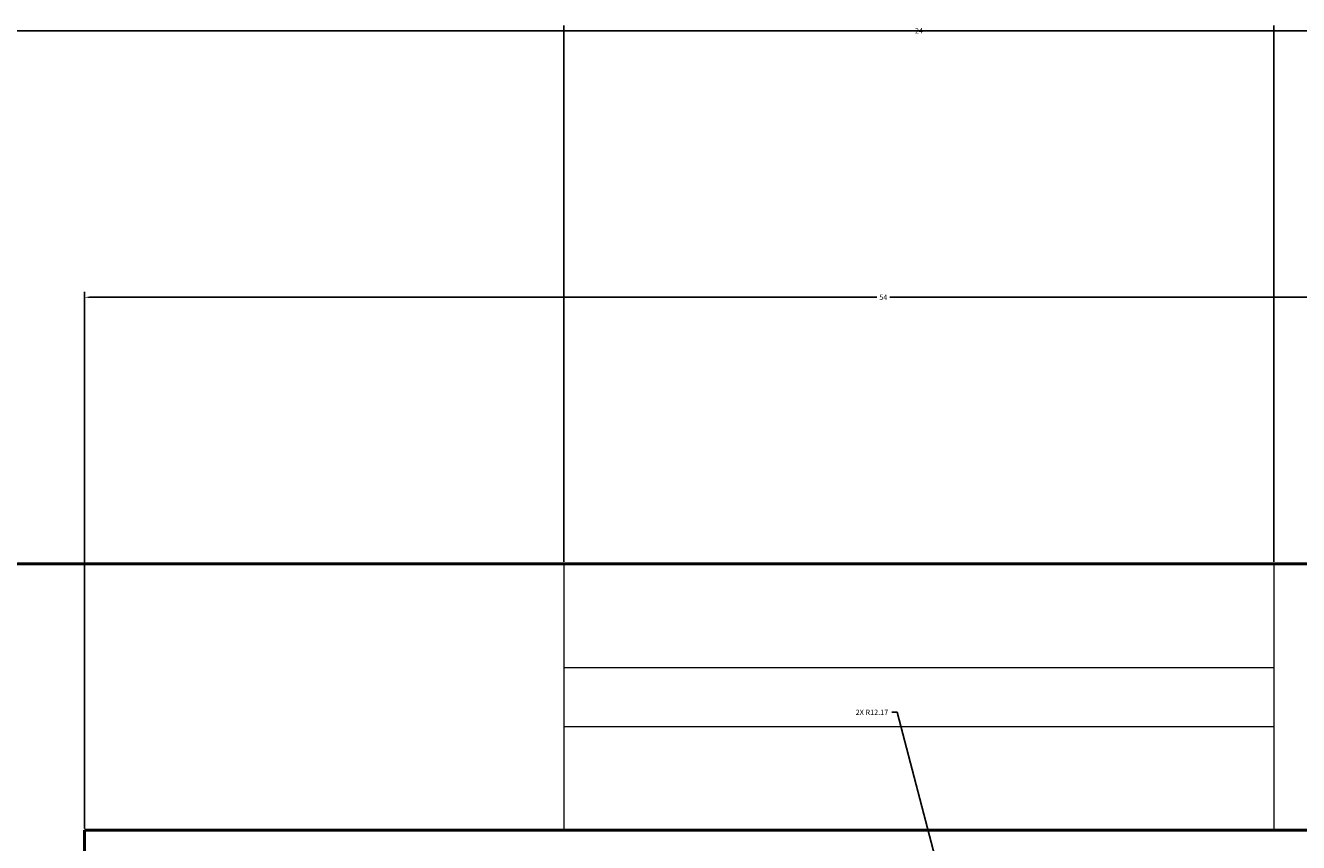
# Model space of a CAD drawing. Units: inches. Extents: x 2621 to 2849, y 2066 to 2463.
# Tile 26 of 28: x 2766 to 2809, y 2435 to 2463. Entities that reach past the tile are written whole.
import ezdxf

# ---------------------------------------------------------------- set-up
doc = ezdxf.new("R2010")
doc.units = ezdxf.units.IN
for name, color, linetype, lineweight in [('A-ANNO-DIMS', 2, 'Continuous', 18), ('A-GLAZ', 4, 'Continuous', 18), ('A-WALL', 7, 'Continuous', 50)]:
    doc.layers.add(name, color=color, linetype=linetype, lineweight=lineweight)
doc.styles.get("Standard").update_dxf_attribs({"font": 'arial.ttf'})
doc.dimstyles.get("Standard").update_dxf_attribs({"dimtxt": 0.18, "dimasz": 0.18, "dimexe": 0.18, "dimexo": 0.0625, "dimgap": 0.09, "dimtad": 0, "dimtih": 1, "dimtoh": 1, "dimdec": 4, "dimzin": 0, "dimdsep": 46, "dimtxsty": 'Standard', "dimcen": 0.09, "dimadec": 0, "dimazin": 0, "dimtfac": 1, "dimtdec": 4, "dimtofl": 0, "dimtmove": 0, "dimatfit": 3, "dimfxl": 1, "dimtolj": 1, "dimtzin": 0, "dimarcsym": 0})

# ---------------------------------------------------------------- blocks, each defined once
blk = doc.blocks.new('*D35')
at = {"layer": 'A-ANNO-DIMS', "color": 0, "lineweight": -2, "transparency": 16777216}
for p, q in [((2638.87, 2444.437), (2638.87, 2462.558)), ((2639.05, 2462.378), (2734.591, 2462.378)), ((2830.69, 2462.378), (2735.15, 2462.378)), ((2830.87, 2444.437), (2830.87, 2462.558))]:
    blk.add_line(p, q, dxfattribs=at)
at = {"layer": 'A-ANNO-DIMS', "color": 0, "transparency": 16777216}
for points in [[(2639.05, 2462.408), (2639.05, 2462.348), (2638.87, 2462.378)], [(2830.69, 2462.408), (2830.69, 2462.348), (2830.87, 2462.378)]]:
    blk.add_solid(points, dxfattribs=at)
at = {"layer": 'Defpoints', "color": 0, "transparency": 16777216}
for p in [(2830.87, 2462.378), (2638.87, 2444.375), (2830.87, 2444.375)]:
    blk.add_point(p, dxfattribs=at)
at = {"layer": 'A-ANNO-DIMS', "color": 0, "transparency": 16777216, "insert": (2734.87, 2462.378), "char_height": 0.18, "attachment_point": 5}
blk.add_mtext('\\A1;192', dxfattribs=at)
blk = doc.blocks.new('*D38')
at = {"layer": 'A-ANNO-DIMS', "color": 0, "lineweight": -2, "transparency": 16777216}
for p, q in [((2784.076, 2444.437), (2784.076, 2462.558)), ((2784.256, 2462.378), (2795.856, 2462.378)), ((2807.896, 2462.378), (2796.296, 2462.378)), ((2808.076, 2444.437), (2808.076, 2462.558))]:
    blk.add_line(p, q, dxfattribs=at)
at = {"layer": 'A-ANNO-DIMS', "color": 0, "transparency": 16777216}
for points in [[(2784.256, 2462.408), (2784.256, 2462.348), (2784.076, 2462.378)], [(2807.896, 2462.408), (2807.896, 2462.348), (2808.076, 2462.378)]]:
    blk.add_solid(points, dxfattribs=at)
at = {"layer": 'Defpoints', "color": 0, "transparency": 16777216}
for p in [(2808.076, 2462.378), (2784.076, 2444.375), (2808.076, 2444.375)]:
    blk.add_point(p, dxfattribs=at)
at = {"layer": 'A-ANNO-DIMS', "color": 0, "transparency": 16777216, "insert": (2796.076, 2462.378), "char_height": 0.18, "attachment_point": 5}
blk.add_mtext('\\A1;24', dxfattribs=at)
blk = doc.blocks.new('*D39')
at = {"layer": 'A-ANNO-DIMS', "color": 0, "lineweight": -2, "transparency": 16777216}
for p, q in [((2808.076, 2444.437), (2808.076, 2462.558)), ((2808.256, 2462.378), (2819.008, 2462.378)), ((2830.69, 2462.378), (2819.938, 2462.378)), ((2830.87, 2444.437), (2830.87, 2462.558))]:
    blk.add_line(p, q, dxfattribs=at)
at = {"layer": 'A-ANNO-DIMS', "color": 0, "transparency": 16777216}
for points in [[(2808.256, 2462.408), (2808.256, 2462.348), (2808.076, 2462.378)], [(2830.69, 2462.408), (2830.69, 2462.348), (2830.87, 2462.378)]]:
    blk.add_solid(points, dxfattribs=at)
at = {"layer": 'Defpoints', "color": 0, "transparency": 16777216}
for p in [(2830.87, 2462.378), (2808.076, 2444.375), (2830.87, 2444.375)]:
    blk.add_point(p, dxfattribs=at)
at = {"layer": 'A-ANNO-DIMS', "color": 0, "transparency": 16777216, "insert": (2819.473, 2462.378), "char_height": 0.18, "attachment_point": 5}
blk.add_mtext('\\A1;22.794', dxfattribs=at)
blk = doc.blocks.new('*D47')
at = {"layer": 'A-ANNO-DIMS', "color": 0, "lineweight": -2, "transparency": 16777216}
for p, q in [((2767.87, 2435.437), (2767.87, 2453.558)), ((2768.05, 2453.378), (2794.652, 2453.378)), ((2821.69, 2453.378), (2795.089, 2453.378)), ((2821.87, 2435.437), (2821.87, 2453.558))]:
    blk.add_line(p, q, dxfattribs=at)
at = {"layer": 'A-ANNO-DIMS', "color": 0, "transparency": 16777216}
for points in [[(2768.05, 2453.408), (2768.05, 2453.348), (2767.87, 2453.378)], [(2821.69, 2453.408), (2821.69, 2453.348), (2821.87, 2453.378)]]:
    blk.add_solid(points, dxfattribs=at)
at = {"layer": 'Defpoints', "color": 0, "transparency": 16777216}
for p in [(2821.87, 2453.378), (2767.87, 2435.375), (2821.87, 2435.375)]:
    blk.add_point(p, dxfattribs=at)
at = {"layer": 'A-ANNO-DIMS', "color": 0, "transparency": 16777216, "insert": (2794.87, 2453.378), "char_height": 0.18, "attachment_point": 5}
blk.add_mtext('\\A1;54', dxfattribs=at)
blk = doc.blocks.new('*D71')
at = {"layer": 'A-ANNO-DIMS', "color": 0, "lineweight": -2, "transparency": 16777216}
for p, q in [((2795.161, 2439.358), (2795.341, 2439.358)), ((2795.341, 2439.358), (2797.151, 2432.47)), ((2800.2, 2420.527), (2800.38, 2420.527)), ((2800.29, 2420.437), (2800.29, 2420.617))]:
    blk.add_line(p, q, dxfattribs=at)
at = {"layer": 'A-ANNO-DIMS', "color": 0, "transparency": 16777216}
blk.add_solid([(2797.18, 2432.478), (2797.122, 2432.463), (2797.197, 2432.296)], dxfattribs=at)
at = {"layer": 'Defpoints', "color": 0, "transparency": 16777216}
for p in [(2797.197, 2432.296), (2800.29, 2420.527)]:
    blk.add_point(p, dxfattribs=at)
at = {"layer": 'A-ANNO-DIMS', "color": 0, "transparency": 16777216, "insert": (2794.487, 2439.358), "char_height": 0.18, "attachment_point": 5}
blk.add_mtext('\\A1;2X R12.17', dxfattribs=at)

msp = doc.modelspace()

# ---------------------------------------------------------------- linework, layer by layer
at = {"layer": 'A-GLAZ'}
for p, q in [((2784.0762, 2440.8746), (2808.0762, 2440.8746)), ((2784.0762, 2438.8746), (2808.0762, 2438.8746))]:
    msp.add_line(p, q, dxfattribs=at)
for points in [[(2784.0762, 2435.3746), (2784.0762, 2444.3746)], [(2808.0762, 2444.3746), (2808.0762, 2435.3746)]]:
    msp.add_lwpolyline(points, dxfattribs=at)
at = {"layer": 'A-WALL'}
for p, q in [((2767.8701, 2435.3746), (2821.8701, 2435.3746)), ((2767.8701, 2375.3746), (2767.8701, 2435.3746))]:
    msp.add_line(p, q, dxfattribs=at)
msp.add_lwpolyline([(2761.8701, 2084.3746), (2638.8701, 2084.3746), (2638.8701, 2444.3746), (2830.8701, 2444.3746), (2830.8701, 2084.3746), (2797.8701, 2084.3746)], dxfattribs=at)

# ---------------------------------------------------------------- dimensions: what is measured, and where the dimension line sits
at = {"layer": 'A-ANNO-DIMS'}
for base, p1, p2, override, picture, middle in [((2830.8701, 2462.3781), (2638.8701, 2444.3746), (2830.8701, 2444.3746), {"dimdec": 0, "dimlfac": 1, "dimrnd": 0, "dimzin": 0, "dimdsep": 46, "dimlunit": 2}, '*D35', (2734.8701, 2462.3781)), ((2808.0762, 2462.3781), (2784.0762, 2444.3746), (2808.0762, 2444.3746), {"dimdec": 0, "dimlfac": 1, "dimrnd": 0, "dimzin": 0, "dimdsep": 46, "dimlunit": 2}, '*D38', (2796.0762, 2462.3781)), ((2830.8701, 2462.3781), (2808.0762, 2444.3746), (2830.8701, 2444.3746), {"dimdec": 3, "dimlfac": 1, "dimrnd": 0, "dimzin": 0, "dimdsep": 46, "dimlunit": 2}, '*D39', (2819.4732, 2462.3781)), ((2821.8701, 2453.3781), (2767.8701, 2435.3746), (2821.8701, 2435.3746), {"dimdec": 0, "dimlfac": 1, "dimrnd": 0, "dimzin": 0, "dimdsep": 46, "dimlunit": 2}, '*D47', (2794.8701, 2453.3781))]:
    dim = msp.add_linear_dim(base=base, p1=p1, p2=p2, dimstyle='Standard', override=override, dxfattribs=at)
    dim.commit()
    dim.dimension.update_dxf_attribs({"geometry": picture, "text_midpoint": middle})
dim = msp.add_radius_dim(center=(2800.2896, 2420.5266), mpoint=(2797.197, 2432.296), text='2X <>', dimstyle='Standard', override={"dimdec": 2, "dimlfac": 1, "dimrnd": 0, "dimzin": 0, "dimdsep": 46, "dimlunit": 2}, dxfattribs=at)
dim.commit()
dim.dimension.update_dxf_attribs({"geometry": '*D71', "text_midpoint": (2794.4867, 2439.3577), "dimtype": 164})

doc.saveas('drawing.dxf')
